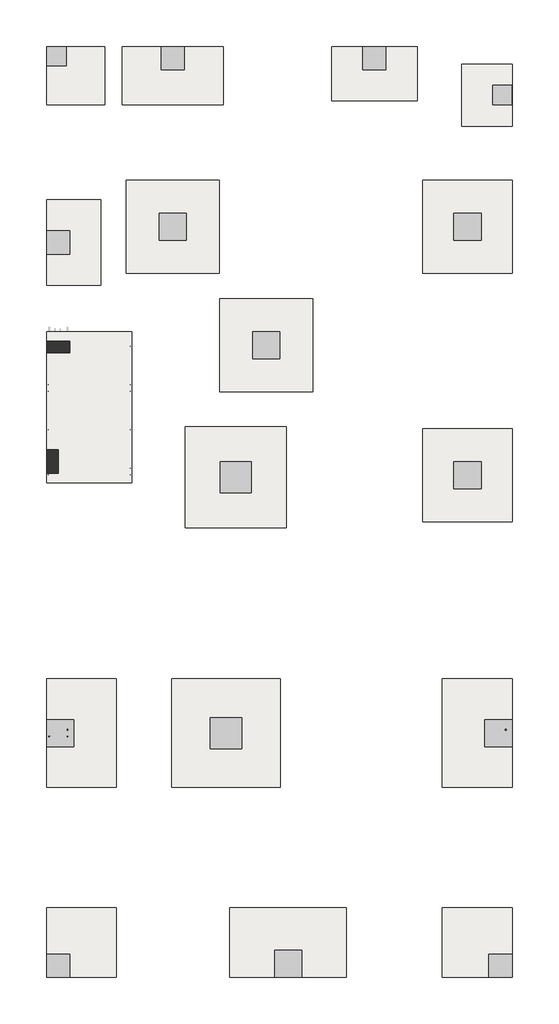
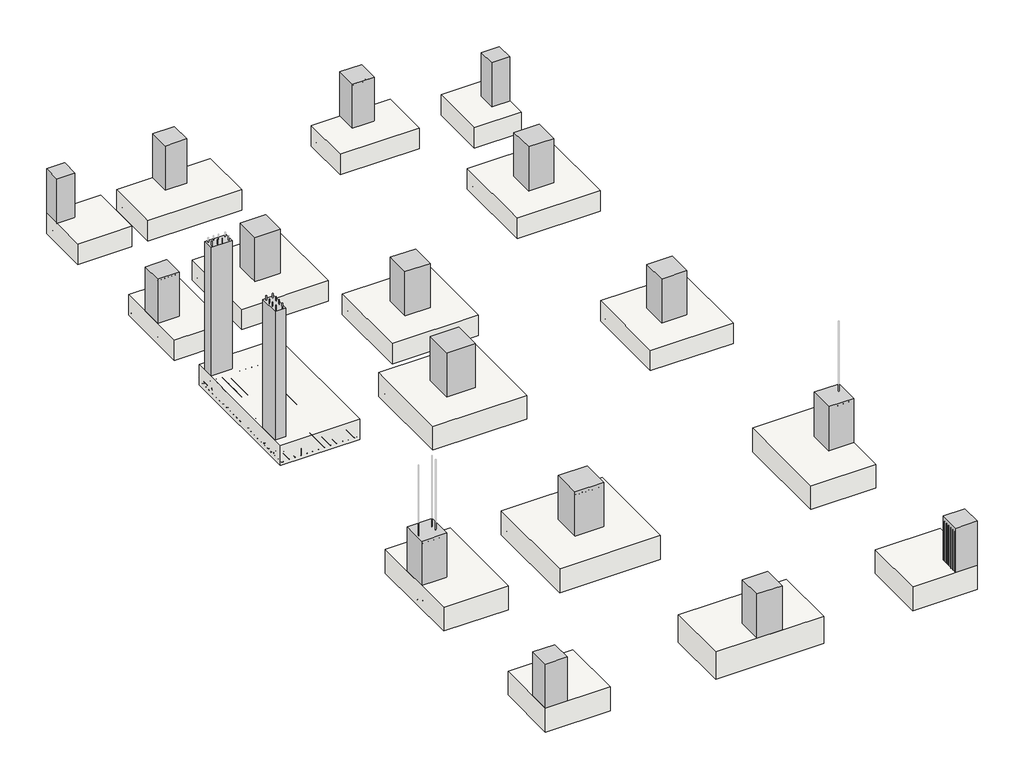
# One storey, part 1 of 6: 18 columns, 17 slabs.
"""IFC4 building model written with IfcOpenShell, lengths in millimetres."""

from ifc_helpers import new_model, si_unit, frame, origin, origin_with_axes, place, context, project, spatial, polyline, outline, extrude, transform, mapped, element, save
from components import concrete_rectangular_column_cf1_9bf53746, concrete_rectangular_column_cf2_4a54b9b5, concrete_rectangular_column_f1_2b960ed8, concrete_rectangular_column_f3_aae16e16, footing_rectangular_cf1_e8ad81a8, footing_rectangular_cf2_90c2f4b8, footing_rectangular_f1_8f1f0fab, footing_rectangular_f2_e38db0b8, footing_rectangular_f3_6d6a3403, footing_rectangular_f4_fcff0cd7, footing_rectangular_lp1_8d3386b4, footing_rectangular_sf1_7ce3103a, footing_rectangular_sf2_5cd490c0, footing_rectangular_sf3_4ecd2a9c, footing_rectangular_sf4_168fb1cd

model = new_model("IFC4")

# Units and contexts
model_context = context("Model", 3, world=origin())
ifc_project = project(units=[si_unit("LENGTHUNIT", "METRE", prefix="MILLI")], contexts=[model_context])

# Site, building, storey
site = spatial("IfcSite", under=ifc_project)
building = spatial("IfcBuilding", under=site)
storey = spatial("IfcBuildingStorey", under=building, Elevation=0.0)

# Columns
placement = place(None, origin())
element("IfcColumn", 1, ObjectType="Concrete-Rectangular-Column : C2", at=placement, inside=storey, context=model_context, shape_type="SweptSolid", body=[
    extrude(outline(polyline([(150274.4232069, -97379.9007776), (150731.6232069, -97379.9007776), (150731.6232069, -97608.5007776), (150274.4232069, -97608.5007776), (150274.4232069, -97379.9007776)])), origin_with_axes(), (0.0, 0.0, 1.0), 2873.0),
])
element("IfcColumn", 2, ObjectType="Concrete-Rectangular-Column : C2", at=placement, inside=storey, context=model_context, shape_type="SweptSolid", body=[
    extrude(outline(polyline([(150503.0232069, -99513.5007776), (150503.0232069, -99970.7007776), (150274.4232069, -99970.7007776), (150274.4232069, -99513.5007776), (150503.0232069, -99513.5007776)])), origin_with_axes(), (0.0, 0.0, 1.0), 2873.0),
])
concrete_rectangular_column_cf1_shape = concrete_rectangular_column_cf1_9bf53746(model_context)
element("IfcColumn", 3, ObjectType="Concrete-Rectangular-Column : CF1", at=placement, inside=storey, context=model_context, shape_type="MappedRepresentation", body=[
    mapped(concrete_rectangular_column_cf1_shape, transform((159189.8232069, -109648.1007776, 0.0), x_axis=(1.0, 0.0, 0.0), y_axis=(0.0, 1.0, 0.0), z_axis=(0.0, 0.0, 1.0))),
])
element("IfcColumn", 4, ObjectType="Concrete-Rectangular-Column : CF1", at=placement, inside=storey, context=model_context, shape_type="MappedRepresentation", body=[
    mapped(concrete_rectangular_column_cf1_shape, transform((150503.0232069, -109648.1007776, 0.0), x_axis=(1.0, 0.0, 0.0), y_axis=(0.0, 1.0, 0.0), z_axis=(0.0, 0.0, 1.0))),
])
concrete_rectangular_column_cf2_shape = concrete_rectangular_column_cf2_4a54b9b5(model_context)
element("IfcColumn", 5, ObjectType="Concrete-Rectangular-Column : CF2", at=placement, inside=storey, context=model_context, shape_type="MappedRepresentation", body=[
    mapped(concrete_rectangular_column_cf2_shape, transform((150464.9232069, -91779.2007776, 0.0), x_axis=(1.0, 0.0, 0.0), y_axis=(0.0, 1.0, 0.0), z_axis=(0.0, 0.0, 1.0))),
])
concrete_rectangular_column_f1_shape = concrete_rectangular_column_f1_2b960ed8(model_context)
element("IfcColumn", 6, ObjectType="Concrete-Rectangular-Column : F1", at=placement, inside=storey, context=model_context, shape_type="MappedRepresentation", body=[
    mapped(concrete_rectangular_column_f1_shape, transform((153798.0805846, -105076.1007776, 0.0), x_axis=(1.0, 0.0, 0.0), y_axis=(0.0, 1.0, 0.0), z_axis=(0.0, 0.0, 1.0))),
])
element("IfcColumn", 7, ObjectType="Concrete-Rectangular-Column : F2", at=placement, inside=storey, context=model_context, shape_type="MappedRepresentation", body=[
    mapped(concrete_rectangular_column_f1_shape, transform((153988.5805846, -100046.9007776, 0.0), x_axis=(1.0, 0.0, 0.0), y_axis=(0.0, 1.0, 0.0), z_axis=(0.0, 0.0, 1.0))),
])
concrete_rectangular_column_f3_shape = concrete_rectangular_column_f3_aae16e16(model_context)
element("IfcColumn", 8, ObjectType="Concrete-Rectangular-Column : F3", at=placement, inside=storey, context=model_context, shape_type="MappedRepresentation", body=[
    mapped(concrete_rectangular_column_f3_shape, transform((152750.9232069, -95132.0007776, 0.0), x_axis=(1.0, 0.0, 0.0), y_axis=(0.0, 1.0, 0.0), z_axis=(0.0, 0.0, 1.0))),
])
element("IfcColumn", 9, ObjectType="Concrete-Rectangular-Column : F3", at=placement, inside=storey, context=model_context, shape_type="MappedRepresentation", body=[
    mapped(concrete_rectangular_column_f3_shape, transform((154585.4805846, -97456.1007776, 0.0), x_axis=(1.0, 0.0, 0.0), y_axis=(0.0, 1.0, 0.0), z_axis=(0.0, 0.0, 1.0))),
])
element("IfcColumn", 10, ObjectType="Concrete-Rectangular-Column : F4", at=placement, inside=storey, context=model_context, shape_type="MappedRepresentation", body=[
    mapped(concrete_rectangular_column_f3_shape, transform((158542.123207, -95132.0007776, 0.0), x_axis=(1.0, 0.0, 0.0), y_axis=(0.0, 1.0, 0.0), z_axis=(0.0, 0.0, 1.0))),
])
element("IfcColumn", 11, ObjectType="Concrete-Rectangular-Column : F4", at=placement, inside=storey, context=model_context, shape_type="MappedRepresentation", body=[
    mapped(concrete_rectangular_column_f3_shape, transform((158542.123207, -100008.8007776, 0.0), x_axis=(1.0, 0.0, 0.0), y_axis=(0.0, 1.0, 0.0), z_axis=(0.0, 0.0, 1.0))),
])
element("IfcColumn", 12, ObjectType="Concrete-Rectangular-Column : SF1", at=placement, inside=storey, context=model_context, shape_type="MappedRepresentation", body=[
    mapped(concrete_rectangular_column_f3_shape, transform((155017.8732069, -109610.0007776, 0.0), x_axis=(1.0, 0.0, 0.0), y_axis=(0.0, 1.0, 0.0), z_axis=(0.0, 0.0, 1.0))),
])
element("IfcColumn", 13, ObjectType="Concrete-Rectangular-Column : SF2", at=placement, inside=storey, context=model_context, shape_type="MappedRepresentation", body=[
    mapped(concrete_rectangular_column_f3_shape, transform((150541.1232069, -105076.1007776, 0.0), x_axis=(1.0, 0.0, 0.0), y_axis=(0.0, 1.0, 0.0), z_axis=(0.0, 0.0, 1.0))),
])
element("IfcColumn", 14, ObjectType="Concrete-Rectangular-Column : SF2", at=placement, inside=storey, context=model_context, shape_type="MappedRepresentation", body=[
    mapped(concrete_rectangular_column_f3_shape, transform((159151.7232069, -105076.1007776, 0.0), x_axis=(1.0, 0.0, 0.0), y_axis=(0.0, 1.0, 0.0), z_axis=(0.0, 0.0, 1.0))),
])
element("IfcColumn", 15, ObjectType="Concrete-Rectangular-Column : SF3", at=placement, inside=storey, context=model_context, shape_type="MappedRepresentation", body=[
    mapped(concrete_rectangular_column_cf1_shape, transform((152750.9232069, -91817.3007776, 0.0), x_axis=(1.0, 0.0, 0.0), y_axis=(0.0, 1.0, 0.0), z_axis=(0.0, 0.0, 1.0))),
])
element("IfcColumn", 16, ObjectType="Concrete-Rectangular-Column : SF4", at=placement, inside=storey, context=model_context, shape_type="MappedRepresentation", body=[
    mapped(concrete_rectangular_column_cf1_shape, transform((156712.8384274, -91817.3007776, 0.0), x_axis=(1.0, 0.0, 0.0), y_axis=(0.0, 1.0, 0.0), z_axis=(0.0, 0.0, 1.0))),
])
element("IfcColumn", 17, ObjectType="Concrete-Rectangular-Column : SF4", at=placement, inside=storey, context=model_context, shape_type="MappedRepresentation", body=[
    mapped(concrete_rectangular_column_cf1_shape, transform((150503.0232069, -95436.8007776, 0.0), x_axis=(1.0, 0.0, 0.0), y_axis=(0.0, 1.0, 0.0), z_axis=(0.0, 0.0, 1.0))),
])
element("IfcColumn", 18, ObjectType="Concrete-Rectangular-Column : SF5", at=placement, inside=storey, context=model_context, shape_type="MappedRepresentation", body=[
    mapped(concrete_rectangular_column_cf2_shape, transform((159225.7937944, -92541.2007776, 0.0), x_axis=(1.0, 0.0, 0.0), y_axis=(0.0, 1.0, 0.0), z_axis=(0.0, 0.0, 1.0))),
])

# Slabs
footing_rectangular_cf1_shape = footing_rectangular_cf1_e8ad81a8(model_context)
element("IfcSlab", 19, ObjectType="Footing-Rectangular : CF1", at=placement, inside=storey, context=model_context, shape_type="MappedRepresentation", body=[
    mapped(footing_rectangular_cf1_shape, transform((150960.2232069, -109190.9007776, 0.0), x_axis=(1.0, 0.0, 0.0), y_axis=(0.0, 1.0, 0.0), z_axis=(0.0, 0.0, 1.0))),
])
element("IfcSlab", 20, ObjectType="Footing-Rectangular : CF1", at=placement, inside=storey, context=model_context, shape_type="MappedRepresentation", body=[
    mapped(footing_rectangular_cf1_shape, transform((158732.6232069, -109190.9007776, 0.0), x_axis=(1.0, 0.0, 0.0), y_axis=(0.0, 1.0, 0.0), z_axis=(0.0, 0.0, 1.0))),
])
footing_rectangular_cf2_shape = footing_rectangular_cf2_90c2f4b8(model_context)
element("IfcSlab", 21, ObjectType="Footing-Rectangular : CF2", at=placement, inside=storey, context=model_context, shape_type="MappedRepresentation", body=[
    mapped(footing_rectangular_cf2_shape, transform((150845.9232069, -92160.2007776, 0.0), x_axis=(1.0, 0.0, 0.0), y_axis=(0.0, 1.0, 0.0), z_axis=(0.0, 0.0, 1.0))),
])
footing_rectangular_f1_shape = footing_rectangular_f1_8f1f0fab(model_context)
element("IfcSlab", 22, ObjectType="Footing-Rectangular : F1", at=placement, inside=storey, context=model_context, shape_type="MappedRepresentation", body=[
    mapped(footing_rectangular_f1_shape, transform((153798.0805846, -105076.1007776, 0.0), x_axis=(1.0, 0.0, 0.0), y_axis=(0.0, 1.0, 0.0), z_axis=(0.0, 0.0, 1.0))),
])
footing_rectangular_f2_shape = footing_rectangular_f2_e38db0b8(model_context)
element("IfcSlab", 23, ObjectType="Footing-Rectangular : F2", at=placement, inside=storey, context=model_context, shape_type="MappedRepresentation", body=[
    mapped(footing_rectangular_f2_shape, transform((153988.5805846, -100046.9007776, 0.0), x_axis=(1.0, 0.0, 0.0), y_axis=(0.0, 1.0, 0.0), z_axis=(0.0, 0.0, 1.0))),
])
footing_rectangular_f3_shape = footing_rectangular_f3_6d6a3403(model_context)
element("IfcSlab", 24, ObjectType="Footing-Rectangular : F3", at=placement, inside=storey, context=model_context, shape_type="MappedRepresentation", body=[
    mapped(footing_rectangular_f3_shape, transform((152750.9232069, -95132.0007776, 0.0), x_axis=(1.0, 0.0, 0.0), y_axis=(0.0, 1.0, 0.0), z_axis=(0.0, 0.0, 1.0))),
])
element("IfcSlab", 25, ObjectType="Footing-Rectangular : F3", at=placement, inside=storey, context=model_context, shape_type="MappedRepresentation", body=[
    mapped(footing_rectangular_f3_shape, transform((154585.4805846, -97456.1317834, 0.0), x_axis=(1.0, 0.0, 0.0), y_axis=(0.0, 1.0, 0.0), z_axis=(0.0, 0.0, 1.0))),
])
element("IfcSlab", 26, ObjectType="Footing-Rectangular : F4", at=placement, inside=storey, context=model_context, shape_type="SweptSolid", body=[
    extrude(outline(polyline([(159418.423207, -94217.6007776), (159418.423207, -96046.4007776), (157665.823207, -96046.4007776), (157665.823207, -94217.6007776), (159418.423207, -94217.6007776)])), frame((0.0, 0.0, -457.2), z_axis=(0.0, 0.0, 1.0), x_axis=(1.0, 0.0, 0.0)), (0.0, 0.0, 1.0), 457.2),
])
footing_rectangular_f4_shape = footing_rectangular_f4_fcff0cd7(model_context)
element("IfcSlab", 27, ObjectType="Footing-Rectangular : F4", at=placement, inside=storey, context=model_context, shape_type="MappedRepresentation", body=[
    mapped(footing_rectangular_f4_shape, transform((158542.123207, -100008.8007776, 0.0), x_axis=(1.0, 0.0, 0.0), y_axis=(0.0, 1.0, 0.0), z_axis=(0.0, 0.0, 1.0))),
])
footing_rectangular_lp1_shape = footing_rectangular_lp1_8d3386b4(model_context)
element("IfcSlab", 28, ObjectType="Footing-Rectangular : LP1", at=placement, inside=storey, context=model_context, shape_type="MappedRepresentation", body=[
    mapped(footing_rectangular_lp1_shape, transform((151112.6232069, -98675.3007776, 0.0), x_axis=(1.0, 0.0, 0.0), y_axis=(0.0, 1.0, 0.0), z_axis=(0.0, 0.0, 1.0))),
])
footing_rectangular_sf1_shape = footing_rectangular_sf1_7ce3103a(model_context)
element("IfcSlab", 29, ObjectType="Footing-Rectangular : SF1", at=placement, inside=storey, context=model_context, shape_type="MappedRepresentation", body=[
    mapped(footing_rectangular_sf1_shape, transform((155017.8732069, -109190.9007776, 0.0), x_axis=(0.0, 1.0, 0.0), y_axis=(-1.0, 0.0, 0.0), z_axis=(0.0, 0.0, 1.0))),
])
footing_rectangular_sf2_shape = footing_rectangular_sf2_5cd490c0(model_context)
element("IfcSlab", 30, ObjectType="Footing-Rectangular : SF2", at=placement, inside=storey, context=model_context, shape_type="MappedRepresentation", body=[
    mapped(footing_rectangular_sf2_shape, transform((150960.2309584, -105076.1162805, 0.0), x_axis=(1.0, 0.0, 0.0), y_axis=(0.0, 1.0, 0.0), z_axis=(0.0, 0.0, 1.0))),
])
element("IfcSlab", 31, ObjectType="Footing-Rectangular : SF2", at=placement, inside=storey, context=model_context, shape_type="MappedRepresentation", body=[
    mapped(footing_rectangular_sf2_shape, transform((158732.6232069, -105076.1007776, 0.0), x_axis=(1.0, 0.0, 0.0), y_axis=(0.0, 1.0, 0.0), z_axis=(0.0, 0.0, 1.0))),
])
footing_rectangular_sf3_shape = footing_rectangular_sf3_4ecd2a9c(model_context)
element("IfcSlab", 32, ObjectType="Footing-Rectangular : SF3", at=placement, inside=storey, context=model_context, shape_type="MappedRepresentation", body=[
    mapped(footing_rectangular_sf3_shape, transform((152750.9232069, -92160.2007776, 0.0), x_axis=(0.0, 1.0, 0.0), y_axis=(-1.0, 0.0, 0.0), z_axis=(0.0, 0.0, 1.0))),
])
footing_rectangular_sf4_shape = footing_rectangular_sf4_168fb1cd(model_context)
element("IfcSlab", 33, ObjectType="Footing-Rectangular : SF4", at=placement, inside=storey, context=model_context, shape_type="MappedRepresentation", body=[
    mapped(footing_rectangular_sf4_shape, transform((156712.8384274, -92122.1007776, 0.0), x_axis=(0.0, 1.0, 0.0), y_axis=(-1.0, 0.0, 0.0), z_axis=(0.0, 0.0, 1.0))),
])
element("IfcSlab", 34, ObjectType="Footing-Rectangular : SF4", at=placement, inside=storey, context=model_context, shape_type="MappedRepresentation", body=[
    mapped(footing_rectangular_sf4_shape, transform((150807.8232069, -95436.8007776, 0.0), x_axis=(1.0, 0.0, 0.0), y_axis=(0.0, 1.0, 0.0), z_axis=(0.0, 0.0, 1.0))),
])
element("IfcSlab", 35, ObjectType="Footing-Rectangular : SF5", at=placement, inside=storey, context=model_context, shape_type="SweptSolid", body=[
    extrude(outline(polyline([(159418.4232069, -91931.6007776), (159418.4232069, -93150.8007776), (158427.8232069, -93150.8007776), (158427.8232069, -91931.6007776), (159418.4232069, -91931.6007776)])), frame((0.0, 0.0, -457.2), z_axis=(0.0, 0.0, 1.0), x_axis=(1.0, 0.0, 0.0)), (0.0, 0.0, 1.0), 457.2),
])

save(model, "model.ifc")

# Revit data of these elements
# Grids (mm)
#   "A": line (150388.723, -90663.29) -> (150388.723, -111076.889)
#   "B": line (152750.923, -90663.29) -> (152750.923, -111076.889)
#   "C": line (153284.323, -90663.29) -> (153284.323, -111076.889)
#   "D": line (153988.581, -90663.29) -> (153988.581, -111076.889)
#   "E": line (155017.873, -90663.29) -> (155017.873, -111076.889)
#   "F": line (156751.423, -90663.29) -> (156751.423, -111076.889)
#   "G": line (158542.123, -90663.29) -> (158542.123, -111076.889)
#   "H": line (159304.123, -90663.29) -> (159304.123, -111076.889)
#   "1": line (149520.846, -109686.201) -> (161515.698, -109686.201)
#   "2": line (149520.846, -105076.101) -> (161515.698, -105076.101)
#   "3": line (149520.846, -99856.401) -> (161515.698, -99856.401)
#   "4": line (149520.846, -97494.201) -> (161515.698, -97494.201)
#   "5": line (149524.923, -95322.501) -> (161515.698, -95322.501)
#   "6": line (161515.698, -92541.201) -> (149520.846, -92541.201)
#   "7": line (149525.11, -91779.201) -> (161515.698, -91779.201)
# Type "Concrete-Rectangular-Column : C2"
#   b = 228.6 mm
#   h = 457.2 mm
#   Structural Material [instance default] = Concrete, Cast-in-Place gray
# Type "Concrete-Rectangular-Column : CF1"
#   b = 457.2 mm
#   h = 457.2 mm
#   Structural Material [instance default] = Concrete, Cast-in-Place gray
# Type "Concrete-Rectangular-Column : CF2"
#   b = 381 mm
#   h = 381 mm
#   Structural Material [instance default] = Concrete, Cast-in-Place gray
# Type "Concrete-Rectangular-Column : F1"
#   b = 609.6 mm
#   h = 609.6 mm
#   Structural Material [instance default] = Concrete, Cast-in-Place gray
# Type "Concrete-Rectangular-Column : F2"
#   b = 609.6 mm
#   h = 609.6 mm
#   Structural Material [instance default] = Concrete, Cast-in-Place gray
# Type "Concrete-Rectangular-Column : F3"
#   b = 533.4 mm
#   h = 533.4 mm
#   Structural Material [instance default] = Concrete, Cast-in-Place gray
# Type "Concrete-Rectangular-Column : F4"
#   b = 533.4 mm
#   h = 533.4 mm
#   Structural Material [instance default] = Concrete, Cast-in-Place gray
# Type "Concrete-Rectangular-Column : SF1"
#   b = 533.4 mm
#   h = 533.4 mm
#   Structural Material [instance default] = Concrete, Cast-in-Place gray
# Type "Concrete-Rectangular-Column : SF2"
#   b = 533.4 mm
#   h = 533.4 mm
#   Structural Material [instance default] = Concrete, Cast-in-Place gray
# Type "Concrete-Rectangular-Column : SF3"
#   b = 457.2 mm
#   h = 457.2 mm
#   Structural Material [instance default] = Concrete, Cast-in-Place gray
# Type "Concrete-Rectangular-Column : SF4"
#   b = 457.2 mm
#   h = 457.2 mm
#   Structural Material [instance default] = Concrete, Cast-in-Place gray
# Type "Concrete-Rectangular-Column : SF5"
#   b = 381 mm
#   h = 381 mm
#   Structural Material [instance default] = Concrete, Cast-in-Place gray
# Type "Footing-Rectangular : CF1"
#   Width = 1371.6 mm
#   Length = 1371.6 mm
#   Foundation Thickness = 533.4 mm
#   Structural Material [instance default] = Concrete - Cast-in-Place Concrete
#   Assembly Code = ""
# Type "Footing-Rectangular : CF2"
#   Width = 1143 mm
#   Length = 1143 mm
#   Foundation Thickness = 457.2 mm
#   Structural Material [instance default] = Concrete - Cast-in-Place Concrete
#   Assembly Code = ""
# Type "Footing-Rectangular : F1"
#   Width = 2133.6 mm
#   Length = 2133.6 mm
#   Foundation Thickness = 533.4 mm
#   Structural Material [instance default] = Concrete - Cast-in-Place Concrete
#   Assembly Code = ""
# Type "Footing-Rectangular : F2"
#   Width = 1981.2 mm
#   Length = 1981.2 mm
#   Foundation Thickness = 533.4 mm
#   Structural Material [instance default] = Concrete - Cast-in-Place Concrete
#   Assembly Code = ""
# Type "Footing-Rectangular : F3"
#   Width = 1828.8 mm
#   Length = 1828.8 mm
#   Foundation Thickness = 457.2 mm
#   Structural Material [instance default] = Concrete - Cast-in-Place Concrete
#   Assembly Code = ""
# Type "Footing-Rectangular : F4"
#   Width = 1752.6 mm
#   Length = 1828.8 mm
#   Foundation Thickness = 457.2 mm
#   Structural Material [instance default] = Concrete - Cast-in-Place Concrete
#   Assembly Code = ""
# Type "Footing-Rectangular : LP1"
#   Width = 1676.4 mm
#   Length = 2971.8 mm
#   Foundation Thickness = 457.2 mm
#   Structural Material [instance default] = Concrete - Cast-in-Place Concrete
#   Assembly Code = ""
# Type "Footing-Rectangular : SF1"
#   Width = 1371.6 mm
#   Length = 2286 mm
#   Foundation Thickness = 609.6 mm
#   Structural Material [instance default] = Concrete - Cast-in-Place Concrete
#   Assembly Code = ""
# Type "Footing-Rectangular : SF2"
#   Width = 1371.6 mm
#   Length = 2133.6 mm
#   Foundation Thickness = 533.4 mm
#   Structural Material [instance default] = Concrete - Cast-in-Place Concrete
#   Assembly Code = ""
# Type "Footing-Rectangular : SF3"
#   Width = 1143 mm
#   Length = 1981.2 mm
#   Foundation Thickness = 457.2 mm
#   Structural Material [instance default] = Concrete - Cast-in-Place Concrete
#   Assembly Code = ""
# Type "Footing-Rectangular : SF4"
#   Width = 1066.8 mm
#   Length = 1676.4 mm
#   Foundation Thickness = 457.2 mm
#   Structural Material [instance default] = Concrete - Cast-in-Place Concrete
#   Assembly Code = ""
# Type "Footing-Rectangular : SF5"
#   Width = 990.6 mm
#   Length = 1219.2 mm
#   Foundation Thickness = 457.2 mm
#   Structural Material [instance default] = Concrete - Cast-in-Place Concrete
#   Assembly Code = ""
# Elements 1, 2 (IfcColumn, "Concrete-Rectangular-Column : C2")
#   Structural Material = Concrete, Cast-in-Place gray
#   Phase Created = New Construction
#   Materials on its faces: "Concrete, Cast-in-Place gray"
# Elements 3, 4 (IfcColumn, "Concrete-Rectangular-Column : CF1")
#   Structural Material = Concrete, Cast-in-Place gray
#   Phase Created = New Construction
#   Materials on its faces: "Concrete, Cast-in-Place gray"
# Element 5 (IfcColumn, "Concrete-Rectangular-Column : CF2")
#   Structural Material = Concrete, Cast-in-Place gray
#   Phase Created = New Construction
#   Materials on its faces: "Concrete, Cast-in-Place gray"
# Element 6 (IfcColumn, "Concrete-Rectangular-Column : F1")
#   Structural Material = Concrete, Cast-in-Place gray
#   Phase Created = New Construction
#   Materials on its faces: "Concrete, Cast-in-Place gray"
# Element 7 (IfcColumn, "Concrete-Rectangular-Column : F2")
#   Structural Material = Concrete, Cast-in-Place gray
#   Phase Created = New Construction
#   Materials on its faces: "Concrete, Cast-in-Place gray"
# Elements 8, 9 (IfcColumn, "Concrete-Rectangular-Column : F3")
#   Structural Material = Concrete, Cast-in-Place gray
#   Phase Created = New Construction
#   Materials on its faces: "Concrete, Cast-in-Place gray"
# Elements 10, 11 (IfcColumn, "Concrete-Rectangular-Column : F4")
#   Structural Material = Concrete, Cast-in-Place gray
#   Phase Created = New Construction
#   Materials on its faces: "Concrete, Cast-in-Place gray"
# Element 12 (IfcColumn, "Concrete-Rectangular-Column : SF1")
#   Structural Material = Concrete, Cast-in-Place gray
#   Phase Created = New Construction
#   Materials on its faces: "Concrete, Cast-in-Place gray"
# Elements 13, 14 (IfcColumn, "Concrete-Rectangular-Column : SF2")
#   Structural Material = Concrete, Cast-in-Place gray
#   Phase Created = New Construction
#   Materials on its faces: "Concrete, Cast-in-Place gray"
# Element 15 (IfcColumn, "Concrete-Rectangular-Column : SF3")
#   Structural Material = Concrete, Cast-in-Place gray
#   Phase Created = New Construction
#   Materials on its faces: "Concrete, Cast-in-Place gray"
# Elements 16, 17 (IfcColumn, "Concrete-Rectangular-Column : SF4")
#   Structural Material = Concrete, Cast-in-Place gray
#   Phase Created = New Construction
#   Materials on its faces: "Concrete, Cast-in-Place gray"
# Element 18 (IfcColumn, "Concrete-Rectangular-Column : SF5")
#   Structural Material = Concrete, Cast-in-Place gray
#   Phase Created = New Construction
#   Materials on its faces: "Concrete, Cast-in-Place gray"
# Elements 19, 20 (IfcSlab, "Footing-Rectangular : CF1")
#   Structural Material = Concrete - Cast-in-Place Concrete
#   Phase Created = New Construction
#   Materials on its faces: "Concrete - Cast-in-Place Concrete"
# Element 21 (IfcSlab, "Footing-Rectangular : CF2")
#   Structural Material = Concrete - Cast-in-Place Concrete
#   Phase Created = New Construction
#   Materials on its faces: "Concrete - Cast-in-Place Concrete"
# Element 22 (IfcSlab, "Footing-Rectangular : F1")
#   Structural Material = Concrete - Cast-in-Place Concrete
#   Phase Created = New Construction
#   Materials on its faces: "Concrete - Cast-in-Place Concrete"
# Element 23 (IfcSlab, "Footing-Rectangular : F2")
#   Structural Material = Concrete - Cast-in-Place Concrete
#   Phase Created = New Construction
#   Materials on its faces: "Concrete - Cast-in-Place Concrete"
# Elements 24, 25 (IfcSlab, "Footing-Rectangular : F3")
#   Structural Material = Concrete - Cast-in-Place Concrete
#   Phase Created = New Construction
#   Materials on its faces: "Concrete - Cast-in-Place Concrete"
# Elements 26, 27 (IfcSlab, "Footing-Rectangular : F4")
#   Structural Material = Concrete - Cast-in-Place Concrete
#   Phase Created = New Construction
#   Materials on its faces: "Concrete - Cast-in-Place Concrete"
# Element 28 (IfcSlab, "Footing-Rectangular : LP1")
#   Structural Material = Concrete - Cast-in-Place Concrete
#   Phase Created = New Construction
#   Materials on its faces: "Concrete - Cast-in-Place Concrete"
# Element 29 (IfcSlab, "Footing-Rectangular : SF1")
#   Structural Material = Concrete - Cast-in-Place Concrete
#   Phase Created = New Construction
#   Materials on its faces: "Concrete - Cast-in-Place Concrete"
# Elements 30, 31 (IfcSlab, "Footing-Rectangular : SF2")
#   Structural Material = Concrete - Cast-in-Place Concrete
#   Phase Created = New Construction
#   Materials on its faces: "Concrete - Cast-in-Place Concrete"
# Element 32 (IfcSlab, "Footing-Rectangular : SF3")
#   Structural Material = Concrete - Cast-in-Place Concrete
#   Phase Created = New Construction
#   Materials on its faces: "Concrete - Cast-in-Place Concrete"
# Elements 33, 34 (IfcSlab, "Footing-Rectangular : SF4")
#   Structural Material = Concrete - Cast-in-Place Concrete
#   Phase Created = New Construction
#   Materials on its faces: "Concrete - Cast-in-Place Concrete"
# Element 35 (IfcSlab, "Footing-Rectangular : SF5")
#   Structural Material = Concrete - Cast-in-Place Concrete
#   Phase Created = New Construction
#   Materials on its faces: "Concrete - Cast-in-Place Concrete"
# Materials
#   "Concrete, Cast-in-Place gray": class "Concrete", colour RGB 192 192 192, transparency 0, Description = "Cast-in-place concrete", Cost = 0
#   "Concrete - Cast-in-Place Concrete": class "Concrete", colour RGB 192 192 192, transparency 0, Cost = 0
